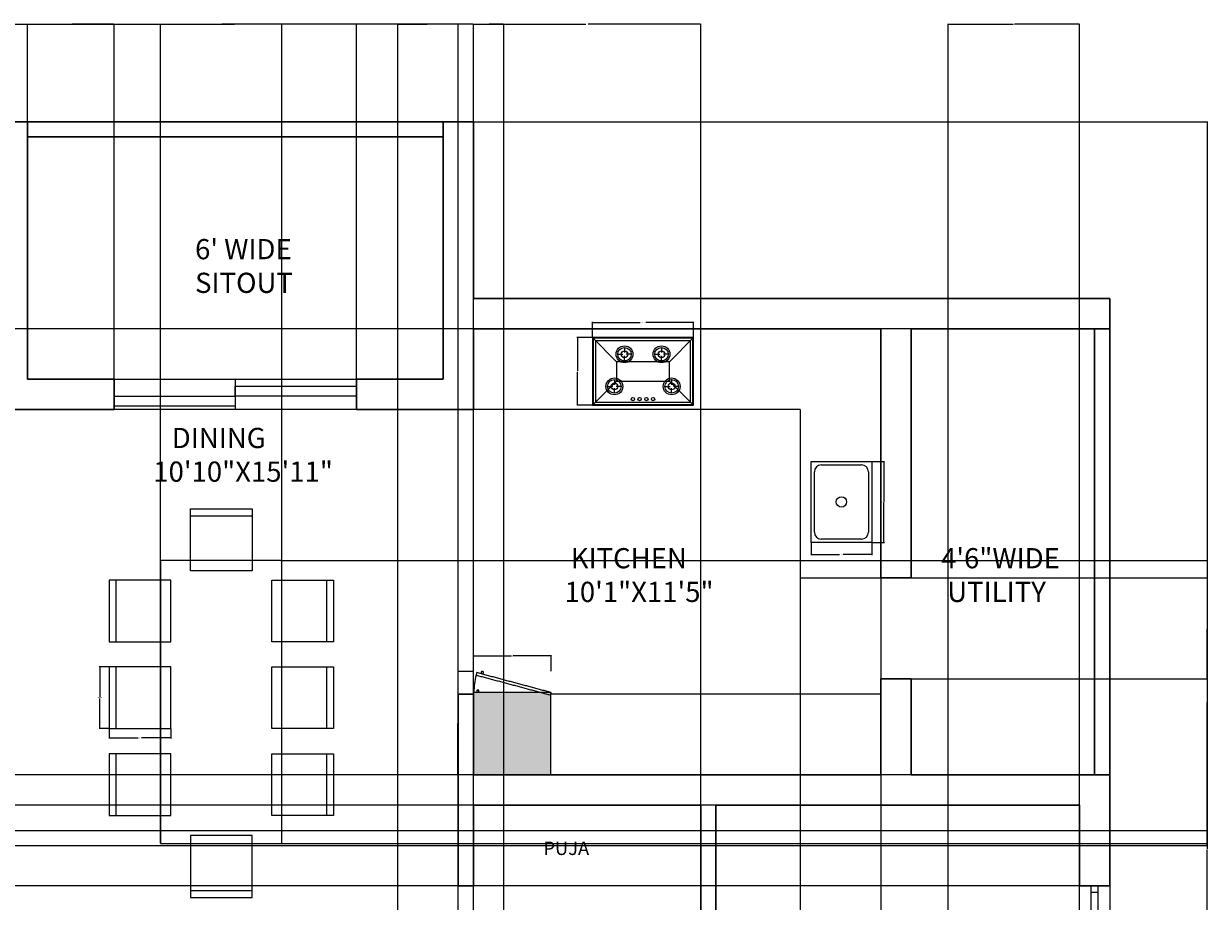
# Model space of a CAD drawing. Units: inches. Extents: x 2134 to 2768, y 715 to 1206.
# Tile 4 of 4: x 2416 to 2768, y 945 to 1206. Entities that reach past the tile are written whole.
import ezdxf

# ---------------------------------------------------------------- set-up
doc = ezdxf.new("R2010")
doc.units = ezdxf.units.IN
for name, color, linetype, lineweight in [('A-ANNO-DIMS', 2, 'Continuous', 18), ('A-AREA-IDEN', 7, 'Continuous', 18), ('A-DOOR', 251, 'Continuous', 13), ('A-EQPM', 9, 'Continuous', 13), ('A-FLOR-CASE', 251, 'Continuous', 13), ('A-FLOR-FIXT', 9, 'Continuous', 13), ('A-FURN', 251, 'Continuous', 13), ('A-WALL', 7, 'Continuous', 30), ('A-WINDOW', 251, 'Continuous', 13), ('Imported blocks', 252, 'Continuous', 9)]:
    doc.layers.add(name, color=color, linetype=linetype, lineweight=lineweight)
doc.styles.get("Standard").update_dxf_attribs({"font": 'arial.ttf'})
doc.dimstyles.get("Standard").update_dxf_attribs({"dimtxt": 0.18, "dimasz": 0.18, "dimexe": 0.18, "dimexo": 0.0625, "dimgap": 0.09, "dimtad": 0, "dimtih": 1, "dimtoh": 1, "dimdec": 4, "dimzin": 0, "dimdsep": 46, "dimtxsty": 'Standard', "dimcen": 0.09, "dimadec": 0, "dimazin": 0, "dimtfac": 1, "dimtdec": 4, "dimtofl": 0, "dimtmove": 0, "dimatfit": 3, "dimfxl": 1, "dimtolj": 1, "dimtzin": 0, "dimarcsym": 0})

# ---------------------------------------------------------------- blocks, each defined once
blk = doc.blocks.new('AN DINIGN CHAIR')
at = {"layer": 'A-FURN', "ltscale": 6}
for p, q in [((6883.8, 1453.73), (6883.8, 1435.73)), ((6901.8, 1453.73), (6883.8, 1453.73)), ((6901.8, 1435.73), (6901.8, 1453.73)), ((6901.8, 1451.73), (6883.8, 1451.73)), ((6883.8, 1435.73), (6901.8, 1435.73))]:
    blk.add_line(p, q, dxfattribs=at)
blk = doc.blocks.new('CHIMNEYU')
at = {"layer": 'A-FURN', "ltscale": 2.5}
for p, q in [((-25.3, 14.2), (-33.3, 22.2)), ((-7.8, 14.2), (0.2, 22.2)), ((-25.3, 7.8), (-33.3, -0.2)), ((-7.8, 7.8), (0.2, -0.2))]:
    blk.add_line(p, q, dxfattribs=at)
for points in [[(-33.3, -0.2), (0.2, -0.2), (0.2, 22.2), (-33.3, 22.2)], [(-33.1, 0), (0, 0), (0, 22), (-33.1, 22)], [(-32.3, 0.8), (-0.8, 0.8), (-0.8, 21.2), (-32.3, 21.2)], [(-25.3, 7.8), (-7.8, 7.8), (-7.8, 14.2), (-25.3, 14.2)]]:
    blk.add_lwpolyline(points, close=True, dxfattribs=at)
blk = doc.blocks.new('stove')
at = {"layer": 'A-FURN'}
for p, q in [((4.46, 14.48), (5.96, 14.48)), ((6.5, 16.48), (6.5, 14.98)), ((8.46, 14.48), (6.96, 14.48)), ((21.46, 14.48), (22.96, 14.48)), ((23.5, 16.48), (23.5, 14.98)), ((25.46, 14.48), (23.96, 14.48)), ((6.5, 12.48), (6.5, 13.98)), ((23.5, 12.48), (23.5, 13.98)), ((7.46, 4.93), (8.96, 4.93)), ((9.5, 6.93), (9.5, 5.43)), ((9.5, 2.93), (9.5, 4.43)), ((11.46, 4.93), (9.96, 4.93)), ((18.46, 4.93), (19.96, 4.93)), ((20.5, 6.93), (20.5, 5.43)), ((20.5, 2.93), (20.5, 4.43)), ((22.46, 4.93), (20.96, 4.93))]:
    blk.add_line(p, q, dxfattribs=at)
for centre, radius in [((12, 18.23), 0.5), ((14, 18.23), 0.5), ((16, 18.23), 0.5), ((18, 18.23), 0.5), ((6.5, 14.48), 2.5), ((6.5, 14.48), 2), ((6.5, 14.48), 1), ((23.5, 14.48), 2.5), ((23.5, 14.48), 2), ((23.5, 14.48), 1), ((9.5, 4.93), 2.5), ((20.5, 4.93), 2.5), ((9.5, 4.93), 2), ((9.5, 4.93), 1), ((20.5, 4.93), 2), ((20.5, 4.93), 1)]:
    blk.add_circle(centre, radius, dxfattribs=at)
at = {"layer": 'A-FURN', "xscale": 0.8955224042543976, "yscale": 0.8955224042543976, "zscale": 0.8955224042543976}
blk.add_blockref('CHIMNEYU', (29.82, 0.18), dxfattribs=at)
blk = doc.blocks.new('sink')
at = {"layer": 'A-FURN'}
for p, q in [((-9, 12), (9, 12)), ((-9, -12), (-9, 12)), ((-6, 11), (6, 11)), ((9, 12), (9, -12)), ((-8, -9), (-8, 9)), ((8, 9), (8, -9)), ((9, -12), (-9, -12)), ((6, -11), (-6, -11))]:
    blk.add_line(p, q, dxfattribs=at)
blk.add_circle((0, 0), 1.53, dxfattribs=at)
for centre, start, end in [((-6, 9), 90, 180), ((6, 9), 0, 90), ((-6, -9), 180, 270), ((6, -9), 270, 0)]:
    blk.add_arc(centre, 2, start, end, dxfattribs=at)
blk = doc.blocks.new("2' ventilators")
at = {"layer": 'A-WINDOW'}
for p, q in [((24, 5.5), (0, 5.5)), ((1.93, 5.5), (1.93, 3.5)), ((22.07, 5.5), (22.07, 3.5))]:
    blk.add_line(p, q, dxfattribs=at)
for points in [[(0, 9), (24, 9), (24, 0), (0, 0), (0, 9)], [(24, 3.5), (0, 3.5)]]:
    blk.add_lwpolyline(points, dxfattribs=at)
blk = doc.blocks.new('Enhet 4')
at = {"layer": 'Imported blocks', "transparency": 33554483}
h = blk.add_hatch(color=256, dxfattribs=at)
edge = h.paths.add_edge_path(flags=0)
edge.add_spline(control_points=[(26.98, 3.49), (27.49, 3.49), (28.01, 3.49)], knot_values=[0, 0, 0, 1, 1, 1], degree=2, periodic=0)
edge.add_spline(control_points=[(28.01, 3.49), (28.01, 16.32), (28.01, 29.16)], knot_values=[0, 0, 0, 1, 1, 1], degree=2, periodic=0)
edge.add_spline(control_points=[(28.01, 29.16), (15.96, 29.16), (3.91, 29.16)], knot_values=[0, 0, 0, 1, 1, 1], degree=2, periodic=0)
edge.add_spline(control_points=[(3.91, 29.16), (3.91, 16.32), (3.91, 3.49)], knot_values=[0, 0, 0, 1, 1, 1], degree=2, periodic=0)
edge.add_spline(control_points=[(3.91, 3.49), (15.13, 3.49), (26.35, 3.49)], knot_values=[0, 0, 0, 1, 1, 1], degree=2, periodic=0)
edge.add_spline(control_points=[(26.35, 3.49), (26.35, 3.12), (26.35, 2.76)], knot_values=[0, 0, 0, 1, 1, 1], degree=2, periodic=0)
edge.add_spline(control_points=[(26.35, 2.76), (26.66, 2.76), (26.98, 2.76)], knot_values=[0, 0, 0, 1, 1, 1], degree=2, periodic=0)
edge.add_spline(control_points=[(26.98, 2.76), (26.98, 3.12), (26.98, 3.49)], knot_values=[0, 0, 0, 1, 1, 1], degree=2, periodic=0)
at = {"layer": 'Imported blocks'}
for points, degree in [([(28.01, 29.16), (15.96, 29.16), (3.91, 29.16)], 2), ([(3.91, 29.16), (3.91, 16.32), (3.91, 3.49)], 2), ([(28.01, 3.49), (28.01, 16.32), (28.01, 29.16)], 2), ([(4, 4.23), (3.91, 3.89), (3.82, 3.55)], 2), ([(4.05, 4.26), (4.01, 4.27), (4, 4.23)], 2), ([(27.15, -1.93), (15.6, 1.16), (4.05, 4.26)], 2), ([(3.82, 3.55), (3.81, 3.51), (3.85, 3.5)], 2), ([(3.85, 3.5), (15.4, 0.4), (26.95, -2.69)], 2), ([(3.91, 3.49), (15.13, 3.49), (26.35, 3.49)], 2), ([(26.35, 3.49), (26.66, 3.49), (26.98, 3.49)], 2), ([(26.35, 3.49), (26.35, 3.12), (26.35, 2.76)], 2), ([(26.35, 2.76), (26.66, 2.76), (26.98, 2.76)], 2), ([(26.98, 3.49), (27.49, 3.49), (28.01, 3.49)], 2), ([(26.98, 2.76), (26.98, 3.12), (26.98, 3.49)], 2), ([(27.18, -1.95), (27.62, -0.17), (27.86, 1.65), (27.89, 3.49)], 3), ([(25.03, -2.18), (24.94, -2.54), (24.84, -2.9)], 2), ([(24.84, -2.9), (25.17, -2.99), (25.51, -3.08)], 2), ([(25.51, -3.08), (25.61, -2.72), (25.7, -2.36)], 2), ([(26.95, -2.69), (26.99, -2.7), (27, -2.66)], 2), ([(27, -2.66), (27.09, -2.32), (27.18, -1.98)], 2), ([(27.18, -1.98), (27.19, -1.94), (27.15, -1.93)], 2)]:
    blk.add_open_spline(points, degree=degree, dxfattribs=at)
blk = doc.blocks.new('*D49')
at = {"layer": 'A-ANNO-DIMS', "color": 0, "lineweight": -2, "transparency": 16777216}
for p, q in [((2441.49, 1014.66), (2438.62, 1014.66)), ((2438.8, 1014.48), (2438.8, 1005.68)), ((2438.8, 996.52), (2438.8, 1005.31)), ((2441.49, 996.34), (2438.62, 996.34))]:
    blk.add_line(p, q, dxfattribs=at)
at = {"layer": 'A-ANNO-DIMS', "color": 0, "transparency": 16777216}
for points in [[(2438.77, 1014.48), (2438.83, 1014.48), (2438.8, 1014.66)], [(2438.77, 996.52), (2438.83, 996.52), (2438.8, 996.34)]]:
    blk.add_solid(points, dxfattribs=at)
at = {"layer": 'Defpoints', "color": 0, "transparency": 16777216}
for p in [(2438.8, 1014.66), (2441.55, 1014.66), (2441.55, 996.34)]:
    blk.add_point(p, dxfattribs=at)
at = {"layer": 'A-ANNO-DIMS', "color": 0, "transparency": 16777216, "insert": (2438.8, 1005.5), "char_height": 0.18, "attachment_point": 5}
blk.add_mtext('\\A1;CHAIR 18 TYP.', dxfattribs=at)
blk = doc.blocks.new('*D50')
at = {"layer": 'A-ANNO-DIMS', "color": 0, "lineweight": -2, "transparency": 16777216}
for p, q in [((2441.55, 996.27), (2441.55, 993.41)), ((2459.87, 996.27), (2459.87, 993.41)), ((2441.73, 993.59), (2450.19, 993.59)), ((2459.69, 993.59), (2451.23, 993.59))]:
    blk.add_line(p, q, dxfattribs=at)
at = {"layer": 'A-ANNO-DIMS', "color": 0, "transparency": 16777216}
for points in [[(2441.73, 993.62), (2441.73, 993.56), (2441.55, 993.59)], [(2459.69, 993.62), (2459.69, 993.56), (2459.87, 993.59)]]:
    blk.add_solid(points, dxfattribs=at)
at = {"layer": 'Defpoints', "color": 0, "transparency": 16777216}
for p in [(2441.55, 996.34), (2459.87, 996.34), (2441.55, 993.59)]:
    blk.add_point(p, dxfattribs=at)
at = {"layer": 'A-ANNO-DIMS', "color": 0, "transparency": 16777216, "insert": (2450.71, 993.59), "char_height": 0.18, "attachment_point": 5}
blk.add_mtext('\\A1;18 TYP.', dxfattribs=at)
blk = doc.blocks.new('*D63')
at = {"layer": 'A-ANNO-DIMS', "color": 0, "lineweight": -2, "transparency": 16777216}
for p, q in [((2668.13, 1075.66), (2671.85, 1075.66)), ((2671.67, 1075.48), (2671.67, 1063.84)), ((2671.67, 1051.84), (2671.67, 1063.48)), ((2668.13, 1051.66), (2671.85, 1051.66))]:
    blk.add_line(p, q, dxfattribs=at)
at = {"layer": 'A-ANNO-DIMS', "color": 0, "transparency": 16777216}
for points in [[(2671.64, 1075.48), (2671.7, 1075.48), (2671.67, 1075.66)], [(2671.64, 1051.84), (2671.7, 1051.84), (2671.67, 1051.66)]]:
    blk.add_solid(points, dxfattribs=at)
at = {"layer": 'Defpoints', "color": 0, "transparency": 16777216}
for p in [(2668.07, 1075.66), (2671.67, 1075.66), (2668.07, 1051.66)]:
    blk.add_point(p, dxfattribs=at)
at = {"layer": 'A-ANNO-DIMS', "color": 0, "transparency": 16777216, "insert": (2671.67, 1063.66), "char_height": 0.18, "attachment_point": 5}
blk.add_mtext('\\A1;SINK 24 TYP.', dxfattribs=at)
blk = doc.blocks.new('*D64')
at = {"layer": 'A-ANNO-DIMS', "color": 0, "lineweight": -2, "transparency": 16777216}
for p, q in [((2650.07, 1051.6), (2650.07, 1047.88)), ((2668.07, 1051.6), (2668.07, 1047.88)), ((2650.25, 1048.06), (2658.55, 1048.06)), ((2667.89, 1048.06), (2659.59, 1048.06))]:
    blk.add_line(p, q, dxfattribs=at)
at = {"layer": 'A-ANNO-DIMS', "color": 0, "transparency": 16777216}
for points in [[(2650.25, 1048.09), (2650.25, 1048.03), (2650.07, 1048.06)], [(2667.89, 1048.09), (2667.89, 1048.03), (2668.07, 1048.06)]]:
    blk.add_solid(points, dxfattribs=at)
at = {"layer": 'Defpoints', "color": 0, "transparency": 16777216}
for p in [(2650.07, 1051.66), (2668.07, 1051.66), (2668.07, 1048.06)]:
    blk.add_point(p, dxfattribs=at)
at = {"layer": 'A-ANNO-DIMS', "color": 0, "transparency": 16777216, "insert": (2659.07, 1048.06), "char_height": 0.18, "attachment_point": 5}
blk.add_mtext('\\A1;18 TYP.', dxfattribs=at)
blk = doc.blocks.new('*D71')
at = {"layer": 'A-ANNO-DIMS', "color": 0, "lineweight": -2, "transparency": 16777216}
for p, q in [((2585.14, 1112.54), (2585.14, 1117.15)), ((2585.32, 1116.97), (2599.26, 1116.97)), ((2614.96, 1116.97), (2601.03, 1116.97)), ((2615.14, 1112.54), (2615.14, 1117.15))]:
    blk.add_line(p, q, dxfattribs=at)
at = {"layer": 'A-ANNO-DIMS', "color": 0, "transparency": 16777216}
for points in [[(2585.32, 1117), (2585.32, 1116.94), (2585.14, 1116.97)], [(2614.96, 1117), (2614.96, 1116.94), (2615.14, 1116.97)]]:
    blk.add_solid(points, dxfattribs=at)
at = {"layer": 'Defpoints', "color": 0, "transparency": 16777216}
for p in [(2585.14, 1116.97), (2585.14, 1112.47), (2615.14, 1112.47)]:
    blk.add_point(p, dxfattribs=at)
at = {"layer": 'A-ANNO-DIMS', "color": 0, "transparency": 16777216, "insert": (2600.14, 1116.97), "char_height": 0.18, "attachment_point": 5}
blk.add_mtext('\\A1;COOKTOP 30', dxfattribs=at)
blk = doc.blocks.new('*D72')
at = {"layer": 'A-ANNO-DIMS', "color": 0, "lineweight": -2, "transparency": 16777216}
for p, q in [((2585.08, 1112.47), (2580.46, 1112.47)), ((2580.64, 1112.29), (2580.64, 1102.63)), ((2580.64, 1092.59), (2580.64, 1102.26)), ((2585.08, 1092.41), (2580.46, 1092.41))]:
    blk.add_line(p, q, dxfattribs=at)
at = {"layer": 'A-ANNO-DIMS', "color": 0, "transparency": 16777216}
for points in [[(2580.61, 1112.29), (2580.67, 1112.29), (2580.64, 1112.47)], [(2580.61, 1092.59), (2580.67, 1092.59), (2580.64, 1092.41)]]:
    blk.add_solid(points, dxfattribs=at)
at = {"layer": 'Defpoints', "color": 0, "transparency": 16777216}
for p in [(2585.14, 1112.47), (2580.64, 1092.41), (2585.14, 1092.41)]:
    blk.add_point(p, dxfattribs=at)
at = {"layer": 'A-ANNO-DIMS', "color": 0, "transparency": 16777216, "insert": (2580.64, 1102.44), "char_height": 0.18, "attachment_point": 5}
blk.add_mtext('\\A1;20', dxfattribs=at)
blk = doc.blocks.new('*D75')
at = {"layer": 'A-ANNO-DIMS', "color": 0, "lineweight": -2, "transparency": 16777216}
for p, q in [((2549.72, 1013.33), (2545, 1013.33)), ((2545.18, 1013.15), (2545.18, 998.14)), ((2545.18, 982.77), (2545.18, 997.78)), ((2549.72, 982.59), (2545, 982.59))]:
    blk.add_line(p, q, dxfattribs=at)
at = {"layer": 'A-ANNO-DIMS', "color": 0, "transparency": 16777216}
for points in [[(2545.15, 1013.15), (2545.21, 1013.15), (2545.18, 1013.33)], [(2545.15, 982.77), (2545.21, 982.77), (2545.18, 982.59)]]:
    blk.add_solid(points, dxfattribs=at)
at = {"layer": 'Defpoints', "color": 0, "transparency": 16777216}
for p in [(2549.79, 1013.33), (2545.18, 982.59), (2549.79, 982.59)]:
    blk.add_point(p, dxfattribs=at)
at = {"layer": 'A-ANNO-DIMS', "color": 0, "transparency": 16777216, "insert": (2545.18, 997.96), "char_height": 0.18, "attachment_point": 5}
blk.add_mtext('\\A1;KITCHEN UNIT 31', dxfattribs=at)
blk = doc.blocks.new('*D76')
at = {"layer": 'A-ANNO-DIMS', "color": 0, "lineweight": -2, "transparency": 16777216}
for p, q in [((2549.79, 1013.39), (2549.79, 1018.12)), ((2549.97, 1017.94), (2561.1, 1017.94)), ((2572.67, 1017.94), (2561.54, 1017.94)), ((2572.85, 1013.39), (2572.85, 1018.12))]:
    blk.add_line(p, q, dxfattribs=at)
at = {"layer": 'A-ANNO-DIMS', "color": 0, "transparency": 16777216}
for points in [[(2549.97, 1017.97), (2549.97, 1017.91), (2549.79, 1017.94)], [(2572.67, 1017.97), (2572.67, 1017.91), (2572.85, 1017.94)]]:
    blk.add_solid(points, dxfattribs=at)
at = {"layer": 'Defpoints', "color": 0, "transparency": 16777216}
for p in [(2549.79, 1017.94), (2549.79, 1013.33), (2572.85, 1013.33)]:
    blk.add_point(p, dxfattribs=at)
at = {"layer": 'A-ANNO-DIMS', "color": 0, "transparency": 16777216, "insert": (2561.32, 1017.94), "char_height": 0.18, "attachment_point": 5}
blk.add_mtext('\\A1;23', dxfattribs=at)
blk = doc.blocks.new('*D78')
at = {"layer": 'A-ANNO-DIMS', "color": 0, "lineweight": -2, "transparency": 16777216}
for p, q in [((2408.29, 1176.67), (2408.29, 1205.74)), ((2408.47, 1205.56), (2478.65, 1205.56)), ((2549.61, 1205.56), (2479.42, 1205.56)), ((2549.79, 1176.67), (2549.79, 1205.74))]:
    blk.add_line(p, q, dxfattribs=at)
at = {"layer": 'A-ANNO-DIMS', "color": 0, "transparency": 16777216}
for points in [[(2408.47, 1205.59), (2408.47, 1205.53), (2408.29, 1205.56)], [(2549.61, 1205.59), (2549.61, 1205.53), (2549.79, 1205.56)]]:
    blk.add_solid(points, dxfattribs=at)
at = {"layer": 'Defpoints', "color": 0, "transparency": 16777216}
for p in [(2549.79, 1205.56), (2408.29, 1176.61), (2549.79, 1176.61)]:
    blk.add_point(p, dxfattribs=at)
at = {"layer": 'A-ANNO-DIMS', "color": 0, "transparency": 16777216, "insert": (2479.04, 1205.56), "char_height": 0.18, "attachment_point": 5}
blk.add_mtext('\\A1;141.5', dxfattribs=at)
blk = doc.blocks.new('*D84')
at = {"layer": 'A-ANNO-DIMS', "color": 0, "lineweight": -2, "transparency": 16777216}
for p, q in [((2527.29, 753.17), (2527.29, 1205.74)), ((2527.47, 1205.56), (2536.08, 1205.56)), ((2545.11, 1205.56), (2536.5, 1205.56)), ((2545.29, 753.17), (2545.29, 1205.74))]:
    blk.add_line(p, q, dxfattribs=at)
at = {"layer": 'A-ANNO-DIMS', "color": 0, "transparency": 16777216}
for points in [[(2527.47, 1205.59), (2527.47, 1205.53), (2527.29, 1205.56)], [(2545.11, 1205.59), (2545.11, 1205.53), (2545.29, 1205.56)]]:
    blk.add_solid(points, dxfattribs=at)
at = {"layer": 'Defpoints', "color": 0, "transparency": 16777216}
for p in [(2545.29, 1205.56), (2527.29, 753.11), (2545.29, 753.11)]:
    blk.add_point(p, dxfattribs=at)
at = {"layer": 'A-ANNO-DIMS', "color": 0, "transparency": 16777216, "insert": (2536.29, 1205.56), "char_height": 0.18, "attachment_point": 5}
blk.add_mtext('\\A1;18', dxfattribs=at)
blk = doc.blocks.new('*D85')
at = {"layer": 'A-ANNO-DIMS', "color": 0, "lineweight": -2, "transparency": 16777216}
for p, q in [((2549.79, 753.17), (2549.79, 1205.74)), ((2549.97, 1205.56), (2554.14, 1205.56)), ((2558.61, 1205.56), (2554.44, 1205.56)), ((2558.79, 753.17), (2558.79, 1205.74))]:
    blk.add_line(p, q, dxfattribs=at)
at = {"layer": 'A-ANNO-DIMS', "color": 0, "transparency": 16777216}
for points in [[(2549.97, 1205.59), (2549.97, 1205.53), (2549.79, 1205.56)], [(2558.61, 1205.59), (2558.61, 1205.53), (2558.79, 1205.56)]]:
    blk.add_solid(points, dxfattribs=at)
at = {"layer": 'Defpoints', "color": 0, "transparency": 16777216}
for p in [(2558.79, 1205.56), (2549.79, 753.11), (2558.79, 753.11)]:
    blk.add_point(p, dxfattribs=at)
at = {"layer": 'A-ANNO-DIMS', "color": 0, "transparency": 16777216, "insert": (2554.29, 1205.56), "char_height": 0.18, "attachment_point": 5}
blk.add_mtext('\\A1;9', dxfattribs=at)
blk = doc.blocks.new('*D89')
at = {"layer": 'A-ANNO-DIMS', "color": 0, "lineweight": -2, "transparency": 16777216}
for p, q in [((2729.72, 973.61), (2134.66, 973.61)), ((2134.84, 973.43), (2134.84, 961.79)), ((2134.84, 949.79), (2134.84, 961.43)), ((2729.72, 949.61), (2134.66, 949.61))]:
    blk.add_line(p, q, dxfattribs=at)
at = {"layer": 'A-ANNO-DIMS', "color": 0, "transparency": 16777216}
for points in [[(2134.81, 973.43), (2134.87, 973.43), (2134.84, 973.61)], [(2134.81, 949.79), (2134.87, 949.79), (2134.84, 949.61)]]:
    blk.add_solid(points, dxfattribs=at)
at = {"layer": 'Defpoints', "color": 0, "transparency": 16777216}
for p in [(2134.84, 973.61), (2729.79, 973.61), (2729.79, 949.61)]:
    blk.add_point(p, dxfattribs=at)
at = {"layer": 'A-ANNO-DIMS', "color": 0, "transparency": 16777216, "insert": (2134.84, 961.61), "char_height": 0.18, "attachment_point": 5}
blk.add_mtext('\\A1;24', dxfattribs=at)
blk = doc.blocks.new('*D92')
at = {"layer": 'A-ANNO-DIMS', "color": 0, "lineweight": -2, "transparency": 16777216}
for p, q in [((2417.29, 1100.17), (2417.29, 1205.74)), ((2417.47, 1205.56), (2429.77, 1205.56)), ((2442.86, 1205.56), (2430.56, 1205.56)), ((2443.04, 1100.17), (2443.04, 1205.74))]:
    blk.add_line(p, q, dxfattribs=at)
at = {"layer": 'A-ANNO-DIMS', "color": 0, "transparency": 16777216}
for points in [[(2417.47, 1205.59), (2417.47, 1205.53), (2417.29, 1205.56)], [(2442.86, 1205.59), (2442.86, 1205.53), (2443.04, 1205.56)]]:
    blk.add_solid(points, dxfattribs=at)
at = {"layer": 'Defpoints', "color": 0, "transparency": 16777216}
for p in [(2443.04, 1205.56), (2417.29, 1100.11), (2443.04, 1100.11)]:
    blk.add_point(p, dxfattribs=at)
at = {"layer": 'A-ANNO-DIMS', "color": 0, "transparency": 16777216, "insert": (2430.16, 1205.56), "char_height": 0.18, "attachment_point": 5}
blk.add_mtext('\\A1;25.75', dxfattribs=at)
blk = doc.blocks.new('*D93')
at = {"layer": 'A-ANNO-DIMS', "color": 0, "lineweight": -2, "transparency": 16777216}
for p, q in [((2443.04, 1100.17), (2443.04, 1205.74)), ((2443.22, 1205.56), (2478.82, 1205.56)), ((2514.86, 1205.56), (2479.25, 1205.56)), ((2515.04, 1100.17), (2515.04, 1205.74))]:
    blk.add_line(p, q, dxfattribs=at)
at = {"layer": 'A-ANNO-DIMS', "color": 0, "transparency": 16777216}
for points in [[(2443.22, 1205.59), (2443.22, 1205.53), (2443.04, 1205.56)], [(2514.86, 1205.59), (2514.86, 1205.53), (2515.04, 1205.56)]]:
    blk.add_solid(points, dxfattribs=at)
at = {"layer": 'Defpoints', "color": 0, "transparency": 16777216}
for p in [(2515.04, 1205.56), (2443.04, 1100.11), (2515.04, 1100.11)]:
    blk.add_point(p, dxfattribs=at)
at = {"layer": 'A-ANNO-DIMS', "color": 0, "transparency": 16777216, "insert": (2479.04, 1205.56), "char_height": 0.18, "attachment_point": 5}
blk.add_mtext('\\A1;72', dxfattribs=at)
blk = doc.blocks.new('*D94')
at = {"layer": 'A-ANNO-DIMS', "color": 0, "lineweight": -2, "transparency": 16777216}
for p, q in [((2549.79, 973.67), (2549.79, 1205.74)), ((2549.97, 1205.56), (2583.21, 1205.56)), ((2617.11, 1205.56), (2583.86, 1205.56)), ((2617.29, 973.67), (2617.29, 1205.74))]:
    blk.add_line(p, q, dxfattribs=at)
at = {"layer": 'A-ANNO-DIMS', "color": 0, "transparency": 16777216}
for points in [[(2549.97, 1205.59), (2549.97, 1205.53), (2549.79, 1205.56)], [(2617.11, 1205.59), (2617.11, 1205.53), (2617.29, 1205.56)]]:
    blk.add_solid(points, dxfattribs=at)
at = {"layer": 'Defpoints', "color": 0, "transparency": 16777216}
for p in [(2617.29, 1205.56), (2549.79, 973.61), (2617.29, 973.61)]:
    blk.add_point(p, dxfattribs=at)
at = {"layer": 'A-ANNO-DIMS', "color": 0, "transparency": 16777216, "insert": (2583.54, 1205.56), "char_height": 0.18, "attachment_point": 5}
blk.add_mtext('\\A1;67.5', dxfattribs=at)
blk = doc.blocks.new('*D95')
at = {"layer": 'A-ANNO-DIMS', "color": 0, "lineweight": -2, "transparency": 16777216}
for p, q in [((2549.72, 973.61), (2134.66, 973.61)), ((2134.84, 973.43), (2134.84, 961.79)), ((2134.84, 949.79), (2134.84, 961.43)), ((2549.72, 949.61), (2134.66, 949.61))]:
    blk.add_line(p, q, dxfattribs=at)
at = {"layer": 'A-ANNO-DIMS', "color": 0, "transparency": 16777216}
for points in [[(2134.81, 973.43), (2134.87, 973.43), (2134.84, 973.61)], [(2134.81, 949.79), (2134.87, 949.79), (2134.84, 949.61)]]:
    blk.add_solid(points, dxfattribs=at)
at = {"layer": 'Defpoints', "color": 0, "transparency": 16777216}
for p in [(2549.79, 973.61), (2134.84, 949.61), (2549.79, 949.61)]:
    blk.add_point(p, dxfattribs=at)
at = {"layer": 'A-ANNO-DIMS', "color": 0, "transparency": 16777216, "insert": (2134.84, 961.61), "char_height": 0.18, "attachment_point": 5}
blk.add_mtext('\\A1;24', dxfattribs=at)
blk = doc.blocks.new('*D96')
at = {"layer": 'A-ANNO-DIMS', "color": 0, "lineweight": -2, "transparency": 16777216}
for p, q in [((2456.87, 962.31), (2456.87, 1205.74)), ((2457.05, 1205.56), (2474.65, 1205.56)), ((2492.69, 1205.56), (2475.09, 1205.56)), ((2492.87, 962.31), (2492.87, 1205.74))]:
    blk.add_line(p, q, dxfattribs=at)
at = {"layer": 'A-ANNO-DIMS', "color": 0, "transparency": 16777216}
for points in [[(2457.05, 1205.59), (2457.05, 1205.53), (2456.87, 1205.56)], [(2492.69, 1205.59), (2492.69, 1205.53), (2492.87, 1205.56)]]:
    blk.add_solid(points, dxfattribs=at)
at = {"layer": 'Defpoints', "color": 0, "transparency": 16777216}
for p in [(2492.87, 1205.56), (2456.87, 962.25), (2492.87, 962.25)]:
    blk.add_point(p, dxfattribs=at)
at = {"layer": 'A-ANNO-DIMS', "color": 0, "transparency": 16777216, "insert": (2474.87, 1205.56), "char_height": 0.18, "attachment_point": 5}
blk.add_mtext('\\A1;36', dxfattribs=at)
blk = doc.blocks.new('*D97')
at = {"layer": 'A-ANNO-DIMS', "color": 0, "lineweight": -2, "transparency": 16777216}
for p, q in [((2492.93, 1046.25), (2767.92, 1046.25)), ((2767.74, 1046.07), (2767.74, 1004.43)), ((2767.74, 962.43), (2767.74, 1004.07)), ((2492.93, 962.25), (2767.92, 962.25))]:
    blk.add_line(p, q, dxfattribs=at)
at = {"layer": 'A-ANNO-DIMS', "color": 0, "transparency": 16777216}
for points in [[(2767.71, 1046.07), (2767.77, 1046.07), (2767.74, 1046.25)], [(2767.71, 962.43), (2767.77, 962.43), (2767.74, 962.25)]]:
    blk.add_solid(points, dxfattribs=at)
at = {"layer": 'Defpoints', "color": 0, "transparency": 16777216}
for p in [(2492.87, 1046.25), (2767.74, 1046.25), (2492.87, 962.25)]:
    blk.add_point(p, dxfattribs=at)
at = {"layer": 'A-ANNO-DIMS', "color": 0, "transparency": 16777216, "insert": (2767.74, 1004.25), "char_height": 0.18, "attachment_point": 5}
blk.add_mtext('\\A1;84', dxfattribs=at)
blk = doc.blocks.new('*D98')
at = {"layer": 'A-ANNO-DIMS', "color": 0, "lineweight": -2, "transparency": 16777216}
for p, q in [((2646.79, 1041.03), (2646.79, 714.98)), ((2670.79, 1041.03), (2670.79, 714.98)), ((2646.97, 715.16), (2658.57, 715.16)), ((2670.61, 715.16), (2659.01, 715.16))]:
    blk.add_line(p, q, dxfattribs=at)
at = {"layer": 'A-ANNO-DIMS', "color": 0, "transparency": 16777216}
for points in [[(2646.97, 715.19), (2646.97, 715.13), (2646.79, 715.16)], [(2670.61, 715.19), (2670.61, 715.13), (2670.79, 715.16)]]:
    blk.add_solid(points, dxfattribs=at)
at = {"layer": 'Defpoints', "color": 0, "transparency": 16777216}
for p in [(2646.79, 1041.09), (2670.79, 1041.09), (2670.79, 715.16)]:
    blk.add_point(p, dxfattribs=at)
at = {"layer": 'A-ANNO-DIMS', "color": 0, "transparency": 16777216, "insert": (2658.79, 715.16), "char_height": 0.18, "attachment_point": 5}
blk.add_mtext('\\A1;24', dxfattribs=at)
blk = doc.blocks.new('*D99')
at = {"layer": 'A-ANNO-DIMS', "color": 0, "lineweight": -2, "transparency": 16777216}
for p, q in [((2679.85, 1041.09), (2767.92, 1041.09)), ((2767.74, 1040.91), (2767.74, 1026.27)), ((2767.74, 1011.27), (2767.74, 1025.91)), ((2679.85, 1011.09), (2767.92, 1011.09))]:
    blk.add_line(p, q, dxfattribs=at)
at = {"layer": 'A-ANNO-DIMS', "color": 0, "transparency": 16777216}
for points in [[(2767.71, 1040.91), (2767.77, 1040.91), (2767.74, 1041.09)], [(2767.71, 1011.27), (2767.77, 1011.27), (2767.74, 1011.09)]]:
    blk.add_solid(points, dxfattribs=at)
at = {"layer": 'Defpoints', "color": 0, "transparency": 16777216}
for p in [(2679.79, 1041.09), (2767.74, 1041.09), (2679.79, 1011.09)]:
    blk.add_point(p, dxfattribs=at)
at = {"layer": 'A-ANNO-DIMS', "color": 0, "transparency": 16777216, "insert": (2767.74, 1026.09), "char_height": 0.18, "attachment_point": 5}
blk.add_mtext('\\A1;30', dxfattribs=at)
blk = doc.blocks.new('*D100')
at = {"layer": 'A-ANNO-DIMS', "color": 0, "lineweight": -2, "transparency": 16777216}
for p, q in [((2679.72, 1115.11), (2134.66, 1115.11)), ((2134.84, 1114.93), (2134.84, 1049.03)), ((2134.84, 982.77), (2134.84, 1048.67)), ((2679.72, 982.59), (2134.66, 982.59))]:
    blk.add_line(p, q, dxfattribs=at)
at = {"layer": 'A-ANNO-DIMS', "color": 0, "transparency": 16777216}
for points in [[(2134.81, 1114.93), (2134.87, 1114.93), (2134.84, 1115.11)], [(2134.81, 982.77), (2134.87, 982.77), (2134.84, 982.59)]]:
    blk.add_solid(points, dxfattribs=at)
at = {"layer": 'Defpoints', "color": 0, "transparency": 16777216}
for p in [(2679.79, 1115.11), (2134.84, 982.59), (2679.79, 982.59)]:
    blk.add_point(p, dxfattribs=at)
at = {"layer": 'A-ANNO-DIMS', "color": 0, "transparency": 16777216, "insert": (2134.84, 1048.85), "char_height": 0.18, "attachment_point": 5}
blk.add_mtext('\\A1;132.52', dxfattribs=at)
blk = doc.blocks.new('*D102')
at = {"layer": 'A-ANNO-DIMS', "color": 0, "lineweight": -2, "transparency": 16777216}
for p, q in [((2199.85, 966.11), (2767.92, 966.11)), ((2767.74, 965.93), (2767.74, 964.04)), ((2199.85, 961.61), (2767.92, 961.61)), ((2767.74, 961.79), (2767.74, 963.68))]:
    blk.add_line(p, q, dxfattribs=at)
at = {"layer": 'A-ANNO-DIMS', "color": 0, "transparency": 16777216}
for points in [[(2767.71, 965.93), (2767.77, 965.93), (2767.74, 966.11)], [(2767.71, 961.79), (2767.77, 961.79), (2767.74, 961.61)]]:
    blk.add_solid(points, dxfattribs=at)
at = {"layer": 'Defpoints', "color": 0, "transparency": 16777216}
for p in [(2199.79, 966.11), (2767.74, 966.11), (2199.79, 961.61)]:
    blk.add_point(p, dxfattribs=at)
at = {"layer": 'A-ANNO-DIMS', "color": 0, "transparency": 16777216, "insert": (2767.74, 963.86), "char_height": 0.18, "attachment_point": 5}
blk.add_mtext('\\A1;4.5', dxfattribs=at)
blk = doc.blocks.new('*D104')
at = {"layer": 'A-ANNO-DIMS', "color": 0, "lineweight": -2, "transparency": 16777216}
for p, q in [((2690.79, 901.67), (2690.79, 1205.74)), ((2690.97, 1205.56), (2710.07, 1205.56)), ((2729.61, 1205.56), (2710.51, 1205.56)), ((2729.79, 901.67), (2729.79, 1205.74))]:
    blk.add_line(p, q, dxfattribs=at)
at = {"layer": 'A-ANNO-DIMS', "color": 0, "transparency": 16777216}
for points in [[(2690.97, 1205.59), (2690.97, 1205.53), (2690.79, 1205.56)], [(2729.61, 1205.59), (2729.61, 1205.53), (2729.79, 1205.56)]]:
    blk.add_solid(points, dxfattribs=at)
at = {"layer": 'Defpoints', "color": 0, "transparency": 16777216}
for p in [(2729.79, 1205.56), (2690.79, 901.61), (2729.79, 901.61)]:
    blk.add_point(p, dxfattribs=at)
at = {"layer": 'A-ANNO-DIMS', "color": 0, "transparency": 16777216, "insert": (2710.29, 1205.56), "char_height": 0.18, "attachment_point": 5}
blk.add_mtext('\\A1;39', dxfattribs=at)
blk = doc.blocks.new('*D106')
at = {"layer": 'A-ANNO-DIMS', "color": 0, "lineweight": -2, "transparency": 16777216}
for p, q in [((2549.85, 1176.61), (2767.92, 1176.61)), ((2767.74, 1176.43), (2767.74, 960.54)), ((2767.74, 744.29), (2767.74, 960.18)), ((2738.85, 744.11), (2767.92, 744.11))]:
    blk.add_line(p, q, dxfattribs=at)
at = {"layer": 'A-ANNO-DIMS', "color": 0, "transparency": 16777216}
for points in [[(2767.71, 1176.43), (2767.77, 1176.43), (2767.74, 1176.61)], [(2767.71, 744.29), (2767.77, 744.29), (2767.74, 744.11)]]:
    blk.add_solid(points, dxfattribs=at)
at = {"layer": 'Defpoints', "color": 0, "transparency": 16777216}
for p in [(2549.79, 1176.61), (2767.74, 1176.61), (2738.79, 744.11)]:
    blk.add_point(p, dxfattribs=at)
at = {"layer": 'A-ANNO-DIMS', "color": 0, "transparency": 16777216, "insert": (2767.74, 960.36), "char_height": 0.18, "attachment_point": 5}
blk.add_mtext('\\A1;432.5', dxfattribs=at)

msp = doc.modelspace()

# ---------------------------------------------------------------- linework, layer by layer
at = {"layer": 'A-DOOR'}
msp.add_line((2479.037, 1100.107), (2479.037, 1091.107), dxfattribs=at)
for points in [[(2443.037, 1100.107), (2515.037, 1100.107), (2515.037, 1091.107), (2443.037, 1091.107)], [(2479.037, 1098.107), (2515.037, 1098.107), (2515.037, 1095.107), (2479.037, 1095.107)], [(2443.037, 1095.107), (2479.037, 1095.107), (2479.037, 1092.107), (2443.037, 1092.107)]]:
    msp.add_lwpolyline(points, close=True, dxfattribs=at)
at = {"layer": 'A-FLOR-CASE'}
for p, q in [((2646.787, 1091.107), (2549.787, 1091.107)), ((2646.787, 1091.107), (2646.787, 1041.091)), ((2646.787, 1041.091), (2670.787, 1041.091)), ((2670.787, 1006.591), (2572.764, 1006.591)), ((2617.287, 949.607), (2549.787, 949.607))]:
    msp.add_line(p, q, dxfattribs=at)
at = {"layer": 'A-FURN'}
msp.add_lwpolyline([(2492.87, 962.249), (2492.87, 1046.249), (2456.87, 1046.249), (2456.87, 962.249)], close=True, dxfattribs=at)
at = {"layer": 'A-WALL'}
for p, q in [((2408.287, 1176.607), (2549.787, 1176.607)), ((2417.287, 1176.607), (2417.287, 1100.107)), ((2540.787, 1176.607), (2540.787, 1100.107)), ((2549.787, 1176.607), (2549.787, 1124.107)), ((2417.287, 1172.107), (2540.787, 1172.107)), ((2738.787, 1124.107), (2549.787, 1124.107)), ((2738.787, 1124.107), (2738.787, 949.607)), ((2670.787, 1115.107), (2549.787, 1115.107)), ((2549.787, 1115.107), (2549.787, 1091.107)), ((2670.787, 1115.107), (2670.787, 1041.091)), ((2738.787, 1115.107), (2679.787, 1115.107)), ((2679.787, 1115.107), (2679.787, 1041.091)), ((2734.287, 1115.107), (2734.287, 982.591)), ((2443.037, 1100.107), (2417.287, 1100.107)), ((2443.037, 1100.107), (2443.037, 1091.107)), ((2540.787, 1100.107), (2515.037, 1100.107)), ((2515.037, 1100.107), (2515.037, 1091.107)), ((2443.037, 1091.107), (2412.787, 1091.107)), ((2549.787, 1091.107), (2515.037, 1091.107)), ((2670.787, 1041.091), (2679.787, 1041.091)), ((2670.787, 1011.091), (2670.787, 982.591)), ((2670.787, 1011.091), (2679.787, 1011.091)), ((2679.787, 1011.091), (2679.787, 982.591)), ((2545.287, 1006.591), (2545.287, 949.607)), ((2545.287, 1006.591), (2549.787, 1006.591)), ((2549.787, 1006.591), (2549.787, 982.591)), ((2670.787, 982.591), (2549.787, 982.591)), ((2734.287, 982.591), (2679.787, 982.591)), ((2734.287, 982.591), (2738.787, 982.591)), ((2549.787, 973.607), (2549.787, 949.607)), ((2617.287, 973.607), (2549.787, 973.607)), ((2617.287, 973.607), (2617.287, 901.607)), ((2729.787, 973.607), (2621.787, 973.607)), ((2621.787, 973.607), (2621.787, 901.607)), ((2729.787, 973.607), (2729.787, 949.607)), ((2549.787, 949.607), (2545.287, 949.607)), ((2729.787, 949.607), (2738.787, 949.607))]:
    msp.add_line(p, q, dxfattribs=at)

# ---------------------------------------------------------------- block references
at = {"layer": 'A-EQPM', "rotation": 180}
msp.add_blockref('stove', (2615.144, 1112.473), dxfattribs=at)
at = {"layer": 'A-EQPM', "xscale": 0.9533872738847108, "yscale": 0.9533872738847108, "zscale": 0.7475420850264571, "rotation": 180}
msp.add_blockref('Enhet 4', (2576.49, 1010.393), dxfattribs=at)
at = {"layer": 'A-FLOR-FIXT'}
msp.add_blockref('sink', (2659.07, 1063.661), dxfattribs=at)
at = {"layer": 'A-FURN', "xscale": -1.017832077187696, "yscale": 1.017832077187696, "zscale": 1.017832077187696}
msp.add_blockref('AN DINIGN CHAIR', (9490.583, -418.079), dxfattribs=at)
at = {"layer": 'A-FURN', "yscale": 1.017832077187696, "zscale": 1.017832077187696}
for p, xscale, rotation in [((3921.198, -5984.413), 1.017832077187696, 90.00000000000003), ((1028.542, -5984.413), -1.017832077187696, 270), ((3921.198, -6010.217), 1.017832077187696, 90.00000000000003), ((1028.542, -6010.217), -1.017832077187696, 270), ((3921.198, -6036.012), 1.017832077187696, 90.00000000000003), ((1028.542, -6036.012), -1.017832077187696, 270), ((9490.583, 2425.867), 1.017832077187696, 180)]:
    msp.add_blockref('AN DINIGN CHAIR', p, dxfattribs=dict(at, xscale=xscale, rotation=rotation))
at = {"layer": 'A-WINDOW', "rotation": 270}
msp.add_blockref("2' ventilators", (2729.787, 949.607), dxfattribs=at)

# ---------------------------------------------------------------- texts
at = {"layer": 'A-AREA-IDEN', "attachment_point": 1}
for s, width, insert, char_height in [(" 6' WIDE \\P SITOUT", 92.46075, (2465.274, 1141.762), 6), ('    DINING\\P 10\'10"X15\'11"', 55.72169, (2452.857, 1085.674), 6), ('  KITCHEN\\P 10\'1"X11\'5"', 55.72169, (2575.007, 1049.954), 6), (' 4\'6"WIDE \\P  UTILITY ', 92.46075, (2686.842, 1049.954), 6), (' PUJA', 55.72169, (2569.313, 962.792), 4)]:
    msp.add_mtext_dynamic_manual_height_columns(s, width=width, gutter_width=12.5, heights=[0], dxfattribs=dict(at, insert=insert, char_height=char_height))

# ---------------------------------------------------------------- dimensions: what is measured, and where the dimension line sits
at = {"layer": 'A-ANNO-DIMS'}
for base, p1, p2, override, picture, middle in [((2549.787, 1205.557), (2408.287, 1176.607), (2549.787, 1176.607), {"dimdec": 1, "dimlfac": 1, "dimrnd": 0, "dimzin": 0, "dimdsep": 46, "dimlunit": 2}, '*D78', (2479.037, 1205.557)), ((2443.037, 1205.557), (2417.287, 1100.107), (2443.037, 1100.107), {"dimdec": 2, "dimlfac": 1, "dimrnd": 0, "dimzin": 0, "dimdsep": 46, "dimlunit": 2}, '*D92', (2430.162, 1205.557)), ((2515.037, 1205.557), (2443.037, 1100.107), (2515.037, 1100.107), {"dimdec": 0, "dimlfac": 1, "dimrnd": 0, "dimzin": 0, "dimdsep": 46, "dimlunit": 2}, '*D93', (2479.037, 1205.557)), ((2492.87, 1205.557), (2456.87, 962.249), (2492.87, 962.249), {"dimdec": 0, "dimlfac": 1, "dimrnd": 0, "dimzin": 0, "dimdsep": 46, "dimlunit": 2}, '*D96', (2474.87, 1205.557)), ((2545.287, 1205.557), (2527.287, 753.107), (2545.287, 753.107), {"dimdec": 0, "dimlfac": 1, "dimrnd": 0, "dimzin": 0, "dimdsep": 46, "dimlunit": 2}, '*D84', (2536.287, 1205.557)), ((2558.787, 1205.557), (2549.787, 753.107), (2558.787, 753.107), {"dimdec": 0, "dimlfac": 1, "dimrnd": 0, "dimzin": 0, "dimdsep": 46, "dimlunit": 2}, '*D85', (2554.287, 1205.557)), ((2617.287, 1205.557), (2549.787, 973.607), (2617.287, 973.607), {"dimdec": 1, "dimlfac": 1, "dimrnd": 0, "dimzin": 0, "dimdsep": 46, "dimlunit": 2}, '*D94', (2583.537, 1205.557)), ((2729.787, 1205.557), (2690.787, 901.607), (2729.787, 901.607), {"dimdec": 0, "dimlfac": 1, "dimrnd": 0, "dimzin": 0, "dimdsep": 46, "dimlunit": 2}, '*D104', (2710.287, 1205.557)), ((2670.787, 715.157), (2646.787, 1041.091), (2670.787, 1041.091), {"dimdec": 0, "dimlfac": 1, "dimrnd": 0, "dimzin": 0, "dimdsep": 46, "dimlunit": 2}, '*D98', (2658.787, 715.157))]:
    dim = msp.add_linear_dim(base=base, p1=p1, p2=p2, dimstyle='Standard', override=override, dxfattribs=at)
    dim.commit()
    dim.dimension.update_dxf_attribs({"geometry": picture, "text_midpoint": middle})
for base, p1, p2, angle, override, picture, middle in [((2767.737, 1176.607), (2738.787, 744.107), (2549.787, 1176.607), 90, {"dimdec": 1, "dimlfac": 1, "dimrnd": 0, "dimzin": 0, "dimdsep": 46, "dimlunit": 2}, '*D106', (2767.737, 960.357)), ((2134.837, 982.591), (2679.787, 1115.107), (2679.787, 982.591), 90, {"dimdec": 2, "dimlfac": 1, "dimrnd": 0, "dimzin": 0, "dimdsep": 46, "dimlunit": 2}, '*D100', (2134.837, 1048.849)), ((2580.644, 1092.414), (2585.144, 1112.473), (2585.144, 1092.414), 270, {"dimdec": 0, "dimlfac": 1, "dimrnd": 0, "dimzin": 0, "dimdsep": 46, "dimlunit": 2}, '*D72', (2580.644, 1102.444)), ((2767.737, 1046.249), (2492.87, 962.249), (2492.87, 1046.249), 90, {"dimdec": 0, "dimlfac": 1, "dimrnd": 0, "dimzin": 0, "dimdsep": 46, "dimlunit": 2}, '*D97', (2767.737, 1004.249)), ((2767.737, 1041.091), (2679.787, 1011.091), (2679.787, 1041.091), 90, {"dimdec": 0, "dimlfac": 1, "dimrnd": 0, "dimzin": 0, "dimdsep": 46, "dimlunit": 2}, '*D99', (2767.737, 1026.091)), ((2549.787, 1017.937), (2572.853, 1013.327), (2549.787, 1013.327), 180, {"dimdec": 0, "dimlfac": 1, "dimrnd": 0, "dimzin": 0, "dimdsep": 46, "dimlunit": 2}, '*D76', (2561.32, 1017.937)), ((2134.837, 973.607), (2729.787, 949.607), (2729.787, 973.607), 90, {"dimdec": 0, "dimlfac": 1, "dimrnd": 0, "dimzin": 0, "dimdsep": 46, "dimlunit": 2}, '*D89', (2134.837, 961.607)), ((2134.837, 949.607), (2549.787, 973.607), (2549.787, 949.607), 90, {"dimdec": 0, "dimlfac": 1, "dimrnd": 0, "dimzin": 0, "dimdsep": 46, "dimlunit": 2}, '*D95', (2134.837, 961.607)), ((2767.737, 966.107), (2199.787, 961.607), (2199.787, 966.107), 90, {"dimdec": 1, "dimlfac": 1, "dimrnd": 0, "dimzin": 0, "dimdsep": 46, "dimlunit": 2}, '*D102', (2767.737, 963.857))]:
    dim = msp.add_linear_dim(base=base, p1=p1, p2=p2, angle=angle, dimstyle='Standard', override=override, dxfattribs=at)
    dim.commit()
    dim.dimension.update_dxf_attribs({"geometry": picture, "text_midpoint": middle})
for base, p1, p2, angle, text, picture, middle in [((2585.144, 1116.973), (2615.144, 1112.473), (2585.144, 1112.473), 180, 'COOKTOP <>', '*D71', (2600.144, 1116.973)), ((2671.67, 1075.661), (2668.07, 1051.661), (2668.07, 1075.661), 90, 'SINK <> TYP.', '*D63', (2671.67, 1063.661)), ((2438.801, 1014.656), (2441.549, 996.335), (2441.549, 1014.656), 90, 'CHAIR <> TYP.', '*D49', (2438.801, 1005.496)), ((2545.177, 982.591), (2549.787, 1013.327), (2549.787, 982.591), 270, 'KITCHEN UNIT <>', '*D75', (2545.177, 997.959)), ((2441.549, 993.587), (2459.87, 996.335), (2441.549, 996.335), 180, '<> TYP.', '*D50', (2450.709, 993.587))]:
    dim = msp.add_linear_dim(base=base, p1=p1, p2=p2, angle=angle, text=text, dimstyle='Standard', override={"dimdec": 0, "dimlfac": 1, "dimrnd": 0, "dimzin": 0, "dimdsep": 46, "dimlunit": 2}, dxfattribs=at)
    dim.commit()
    dim.dimension.update_dxf_attribs({"geometry": picture, "text_midpoint": middle})
dim = msp.add_linear_dim(base=(2668.07, 1048.061), p1=(2650.07, 1051.661), p2=(2668.07, 1051.661), text='<> TYP.', dimstyle='Standard', override={"dimdec": 0, "dimlfac": 1, "dimrnd": 0, "dimzin": 0, "dimdsep": 46, "dimlunit": 2}, dxfattribs=at)
dim.commit()
dim.dimension.update_dxf_attribs({"geometry": '*D64', "text_midpoint": (2659.07, 1048.061)})

doc.saveas('drawing.dxf')
